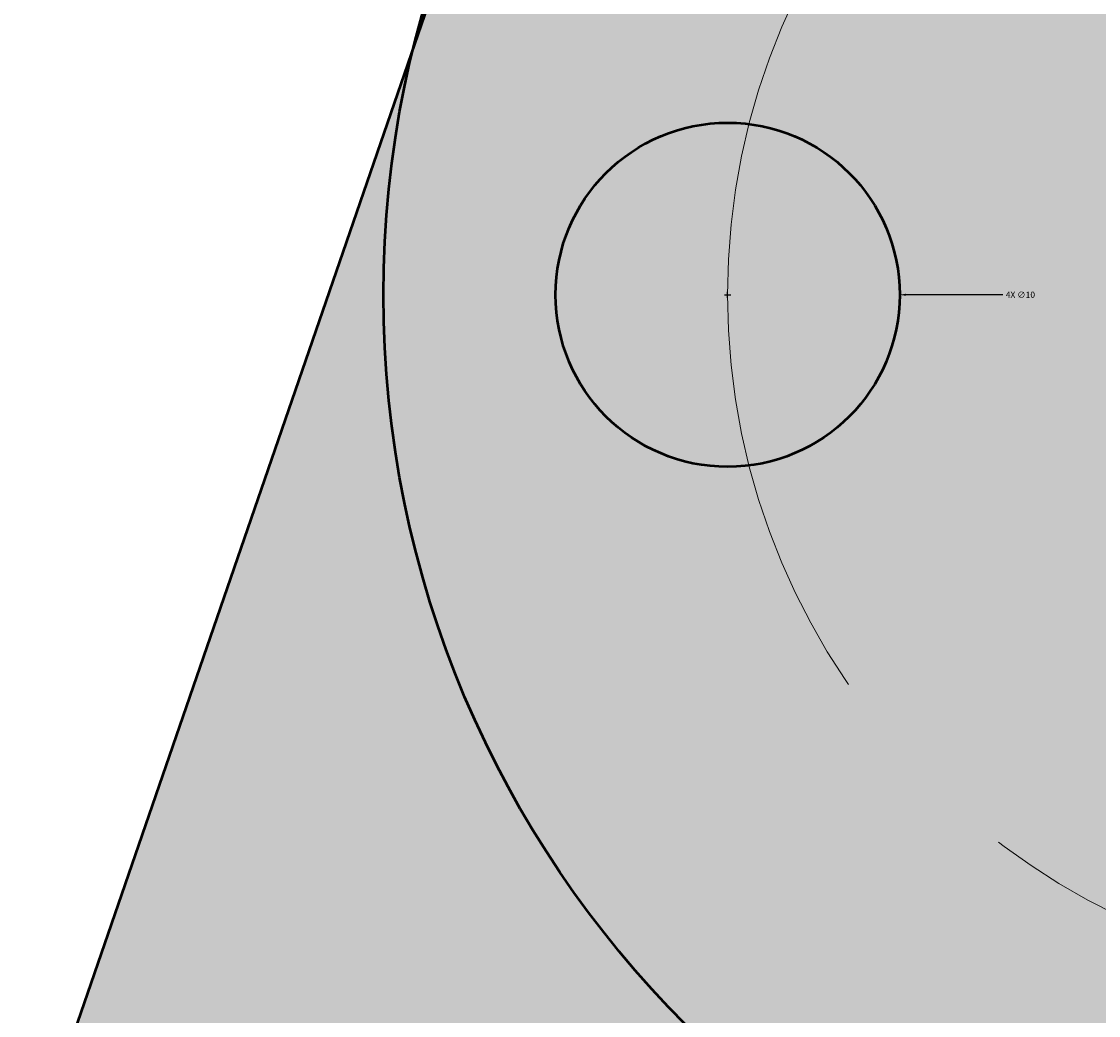
# Model space of a CAD drawing. Units: inches. Extents: x 114 to 236, y -51 to 115.
# Tile 7 of 14: x 135 to 166, y 58 to 87. Entities that reach past the tile are written whole.
import ezdxf

# ---------------------------------------------------------------- set-up
doc = ezdxf.new("R2010")
doc.units = ezdxf.units.IN
doc.header["$MEASUREMENT"] = 0
doc.linetypes.add('CENTER', pattern=[50.8, 31.75, -6.35, 6.35, -6.35])
for name, color, linetype, lineweight in [('M-CNTR', 7, 'CENTER', 18), ('M-DIMS', 2, 'Continuous', 18), ('M-OUTL', 7, 'Continuous', 50)]:
    doc.layers.add(name, color=color, linetype=linetype, lineweight=lineweight)
doc.layers.add('M-HATC', color=7, linetype='Continuous', lineweight=18, true_color=0xffffff)
doc.styles.get("Standard").update_dxf_attribs({"font": 'arial.ttf'})
doc.dimstyles.get("Standard").update_dxf_attribs({"dimtxt": 0.18, "dimasz": 0.18, "dimexe": 0.18, "dimexo": 0.0625, "dimgap": 0.09, "dimtad": 0, "dimtih": 1, "dimtoh": 1, "dimdec": 4, "dimzin": 0, "dimdsep": 46, "dimtxsty": 'Standard', "dimcen": 0.09, "dimadec": 0, "dimazin": 0, "dimtfac": 1, "dimtdec": 4, "dimtofl": 0, "dimtmove": 0, "dimatfit": 3, "dimfxl": 1, "dimtolj": 1, "dimtzin": 0, "dimarcsym": 0})

# ---------------------------------------------------------------- blocks, each defined once
blk = doc.blocks.new('BOLT-HOLE-D10')
blk.add_circle((0, 0), 5)
blk = doc.blocks.new('*D3')
at = {"layer": 'Defpoints', "color": 0, "transparency": 16777216}
for p in [(230.229, 115.287), (120.229, 9.307), (230.229, 9.307)]:
    blk.add_point(p, dxfattribs=at)
at = {"layer": 'M-DIMS', "color": 0, "lineweight": -2, "transparency": 16777216}
for p, q in [((120.229, 9.37), (120.229, 115.467)), ((120.409, 115.287), (174.949, 115.287)), ((230.049, 115.287), (175.509, 115.287)), ((230.229, 9.37), (230.229, 115.467))]:
    blk.add_line(p, q, dxfattribs=at)
at = {"layer": 'M-DIMS', "color": 0, "transparency": 16777216}
for points in [[(120.409, 115.317), (120.409, 115.257), (120.229, 115.287)], [(230.049, 115.317), (230.049, 115.257), (230.229, 115.287)]]:
    blk.add_solid(points, dxfattribs=at)
at = {"layer": 'M-DIMS', "color": 0, "transparency": 16777216, "insert": (175.229, 115.287), "char_height": 0.18, "attachment_point": 5}
blk.add_mtext('\\A1;110', dxfattribs=at)
blk = doc.blocks.new('*D4')
at = {"layer": 'Defpoints', "color": 0, "transparency": 16777216}
for p in [(114.249, 109.307), (175.229, 109.307), (135.229, -5.693)]:
    blk.add_point(p, dxfattribs=at)
at = {"layer": 'M-DIMS', "color": 0, "lineweight": -2, "transparency": 16777216}
for p, q in [((175.166, 109.307), (114.069, 109.307)), ((114.249, 109.127), (114.249, 51.989)), ((114.249, -5.513), (114.249, 51.625)), ((135.166, -5.693), (114.069, -5.693))]:
    blk.add_line(p, q, dxfattribs=at)
at = {"layer": 'M-DIMS', "color": 0, "transparency": 16777216}
for points in [[(114.219, 109.127), (114.279, 109.127), (114.249, 109.307)], [(114.219, -5.513), (114.279, -5.513), (114.249, -5.693)]]:
    blk.add_solid(points, dxfattribs=at)
at = {"layer": 'M-DIMS', "color": 0, "transparency": 16777216, "insert": (114.249, 51.807), "char_height": 0.18, "attachment_point": 5}
blk.add_mtext('\\A1;115', dxfattribs=at)
blk = doc.blocks.new('*D5')
at = {"layer": 'Defpoints', "color": 0, "transparency": 16777216}
for p in [(175.229, 79.307), (135.229, 9.307), (175.229, -11.673)]:
    blk.add_point(p, dxfattribs=at)
at = {"layer": 'M-DIMS', "color": 0, "lineweight": -2, "transparency": 16777216}
for p, q in [((175.229, 79.245), (175.229, -11.853)), ((135.229, 9.245), (135.229, -11.853)), ((135.409, -11.673), (155.006, -11.673)), ((175.049, -11.673), (155.451, -11.673))]:
    blk.add_line(p, q, dxfattribs=at)
at = {"layer": 'M-DIMS', "color": 0, "transparency": 16777216}
for points in [[(135.409, -11.643), (135.409, -11.703), (135.229, -11.673)], [(175.049, -11.643), (175.049, -11.703), (175.229, -11.673)]]:
    blk.add_solid(points, dxfattribs=at)
at = {"layer": 'M-DIMS', "color": 0, "transparency": 16777216, "insert": (155.229, -11.673), "char_height": 0.18, "attachment_point": 5}
blk.add_mtext('\\A1;40', dxfattribs=at)
blk = doc.blocks.new('*D8')
at = {"layer": 'Defpoints', "color": 0, "transparency": 16777216}
for p in [(197.149, 99.789), (153.308, 58.825)]:
    blk.add_point(p, dxfattribs=at)
at = {"layer": 'M-DIMS', "color": 0, "lineweight": -2, "transparency": 16777216}
for p, q in [((210.301, 112.078), (197.28, 99.912)), ((210.481, 112.078), (210.301, 112.078)), ((175.139, 79.307), (175.319, 79.307)), ((175.229, 79.217), (175.229, 79.397))]:
    blk.add_line(p, q, dxfattribs=at)
at = {"layer": 'M-DIMS', "color": 0, "transparency": 16777216}
blk.add_solid([(197.26, 99.934), (197.301, 99.89), (197.149, 99.789)], dxfattribs=at)
at = {"layer": 'M-DIMS', "color": 0, "transparency": 16777216, "insert": (210.797, 112.078), "char_height": 0.18, "attachment_point": 5}
blk.add_mtext('\\A1;∅60', dxfattribs=at)
blk = doc.blocks.new('*D9')
at = {"layer": 'Defpoints', "color": 0, "transparency": 16777216}
for p in [(157.908, 89.307), (192.549, 69.307)]:
    blk.add_point(p, dxfattribs=at)
at = {"layer": 'M-DIMS', "color": 0, "lineweight": -2, "transparency": 16777216}
for p, q in [((147.336, 95.307), (147.516, 95.307)), ((147.516, 95.307), (157.752, 89.397)), ((175.139, 79.307), (175.319, 79.307)), ((175.229, 79.217), (175.229, 79.397))]:
    blk.add_line(p, q, dxfattribs=at)
at = {"layer": 'M-DIMS', "color": 0, "transparency": 16777216}
blk.add_solid([(157.767, 89.423), (157.737, 89.371), (157.908, 89.307)], dxfattribs=at)
at = {"layer": 'M-DIMS', "color": 0, "transparency": 16777216, "insert": (147.019, 95.307), "char_height": 0.18, "attachment_point": 5}
blk.add_mtext('\\A1;∅40', dxfattribs=at)
blk = doc.blocks.new('*D11')
at = {"layer": 'Defpoints', "color": 0, "transparency": 16777216}
for p in [(150.229, 79.307), (160.229, 79.307)]:
    blk.add_point(p, dxfattribs=at)
at = {"layer": 'M-DIMS', "color": 0, "lineweight": -2, "transparency": 16777216}
for p, q in [((155.139, 79.307), (155.319, 79.307)), ((155.229, 79.217), (155.229, 79.397)), ((163.229, 79.307), (160.409, 79.307))]:
    blk.add_line(p, q, dxfattribs=at)
at = {"layer": 'M-DIMS', "color": 0, "transparency": 16777216}
blk.add_solid([(160.409, 79.337), (160.409, 79.277), (160.229, 79.307)], dxfattribs=at)
at = {"layer": 'M-DIMS', "color": 0, "transparency": 16777216, "insert": (163.737, 79.307), "char_height": 0.18, "attachment_point": 5}
blk.add_mtext('\\A1;4X ∅10', dxfattribs=at)

msp = doc.modelspace()

# ---------------------------------------------------------------- hatches: boundary and pattern name
at = {"layer": 'M-HATC'}
h = msp.add_hatch(color=256, dxfattribs=at)
h.set_gradient(color1=(19, 155, 72), color2=(255, 255, 0), tint=1, name='HEMISPHERICAL')
h.paths.add_polyline_path([(147.853, 91.577), (146.105, 86.505, 0.060651), (145.229, 79.307, 1), (205.229, 79.307, 0.060651), (204.352, 86.505), (202.605, 91.577, 0.647643)])
h.paths.add_polyline_path([(180.229, 99.307, -0.031342), (180.189, 98.682, -0.27393), (194.604, 84.268, -0.451416), (200.229, 79.307, -0.451416), (194.604, 74.346, -0.27393), (180.189, 59.932, -0.031342), (180.229, 59.307, -1), (170.229, 59.307, -0.031342), (170.268, 59.932, -0.27393), (155.854, 74.346, -0.451416), (150.229, 79.307, -0.451416), (155.854, 84.268, -0.27393), (170.268, 98.682, -0.031342), (170.229, 99.307, -1)], flags=16)
h.paths.add_polyline_path([(183.229, 79.307, -1), (167.229, 79.307, -1)], flags=0)
h.paths.add_polyline_path([(155.854, 84.268, -0.377964), (160.229, 79.307, -0.377964), (155.854, 74.346, 0.27393), (170.268, 59.932, -0.881917), (180.189, 59.932, 0.27393), (194.604, 74.346, -0.377964), (190.229, 79.307, -0.377964), (194.604, 84.268, 0.27393), (180.189, 98.682, -0.881917), (170.268, 98.682, 0.27393)], flags=0)
h = msp.add_hatch(color=256, dxfattribs=at)
h.set_gradient(color1=(242, 103, 34), color2=(255, 255, 0), tint=1, name='INVSPHERICAL')
h.paths.add_polyline_path([(145.229, 79.307, -0.060651), (146.105, 86.505), (121.823, 16.038, -0.790743), (150.229, 9.307, -0.236068), (144.229, -2.693, -0.14094), (175.229, 9.098, -0.14094), (206.229, -2.693, -0.236068), (200.229, 9.307, -0.790743), (228.634, 16.038), (204.352, 86.505, -0.060651), (205.229, 79.307, -1)])
h = msp.add_hatch(color=256, dxfattribs=at)
h.paths.add_polyline_path([(155.229, 79.307, -0.062746), (155.854, 84.268, 0.451416), (150.229, 79.307, 0.451416), (155.854, 74.346, -0.062746)])
h.paths.add_polyline_path([(155.854, 84.268, 0.062746), (155.229, 79.307, 0.062746), (155.854, 74.346, 0.377964), (160.229, 79.307, 0.377964)])

# ---------------------------------------------------------------- linework, layer by layer
at = {"layer": 'M-CNTR'}
msp.add_circle((175.229, 79.307), 20, dxfattribs=at)
at = {"layer": 'M-OUTL'}
msp.add_line((120.523, 12.263), (147.853, 91.577), dxfattribs=at)
msp.add_circle((175.229, 79.307), 30, dxfattribs=at)

# ---------------------------------------------------------------- block references
msp.add_blockref('BOLT-HOLE-D10', (155.229, 79.307), dxfattribs=at)

# ---------------------------------------------------------------- dimensions: what is measured, and where the dimension line sits
at = {"layer": 'M-DIMS'}
for base, p1, p2, picture, middle in [((230.229, 115.287), (120.229, 9.307), (230.229, 9.307), '*D3', (175.229, 115.287)), ((175.229, -11.673), (135.229, 9.307), (175.229, 79.307), '*D5', (155.229, -11.673))]:
    dim = msp.add_linear_dim(base=base, p1=p1, p2=p2, dimstyle='Standard', override={"dimdec": 0, "dimlfac": 1, "dimrnd": 0, "dimzin": 0, "dimdsep": 46, "dimlunit": 2}, dxfattribs=at)
    dim.commit()
    dim.dimension.update_dxf_attribs({"geometry": picture, "text_midpoint": middle})
for p1, p2, picture, middle in [((153.308, 58.825), (197.149, 99.789), '*D8', (210.797, 112.078)), ((192.549, 69.307), (157.908, 89.307), '*D9', (147.019, 95.307))]:
    dim = msp.add_diameter_dim_2p(p1=p1, p2=p2, dimstyle='Standard', override={"dimdec": 0, "dimlfac": 1, "dimrnd": 0, "dimzin": 0, "dimdsep": 46, "dimlunit": 2}, dxfattribs=at)
    dim.commit()
    dim.dimension.update_dxf_attribs({"geometry": picture, "text_midpoint": middle, "dimtype": 163})
dim = msp.add_linear_dim(base=(114.249, 109.307), p1=(135.229, -5.693), p2=(175.229, 109.307), angle=90, dimstyle='Standard', override={"dimdec": 0, "dimlfac": 1, "dimrnd": 0, "dimzin": 0, "dimdsep": 46, "dimlunit": 2}, dxfattribs=at)
dim.commit()
dim.dimension.update_dxf_attribs({"geometry": '*D4', "text_midpoint": (114.249, 51.807)})
dim = msp.add_diameter_dim_2p(p1=(150.229, 79.307), p2=(160.229, 79.307), text='4X <>', dimstyle='Standard', override={"dimdec": 0, "dimlfac": 1, "dimrnd": 0, "dimzin": 0, "dimdsep": 46, "dimlunit": 2}, dxfattribs=at)
dim.commit()
dim.dimension.update_dxf_attribs({"geometry": '*D11', "text_midpoint": (163.229, 79.307), "dimtype": 163})

doc.saveas('drawing.dxf')
